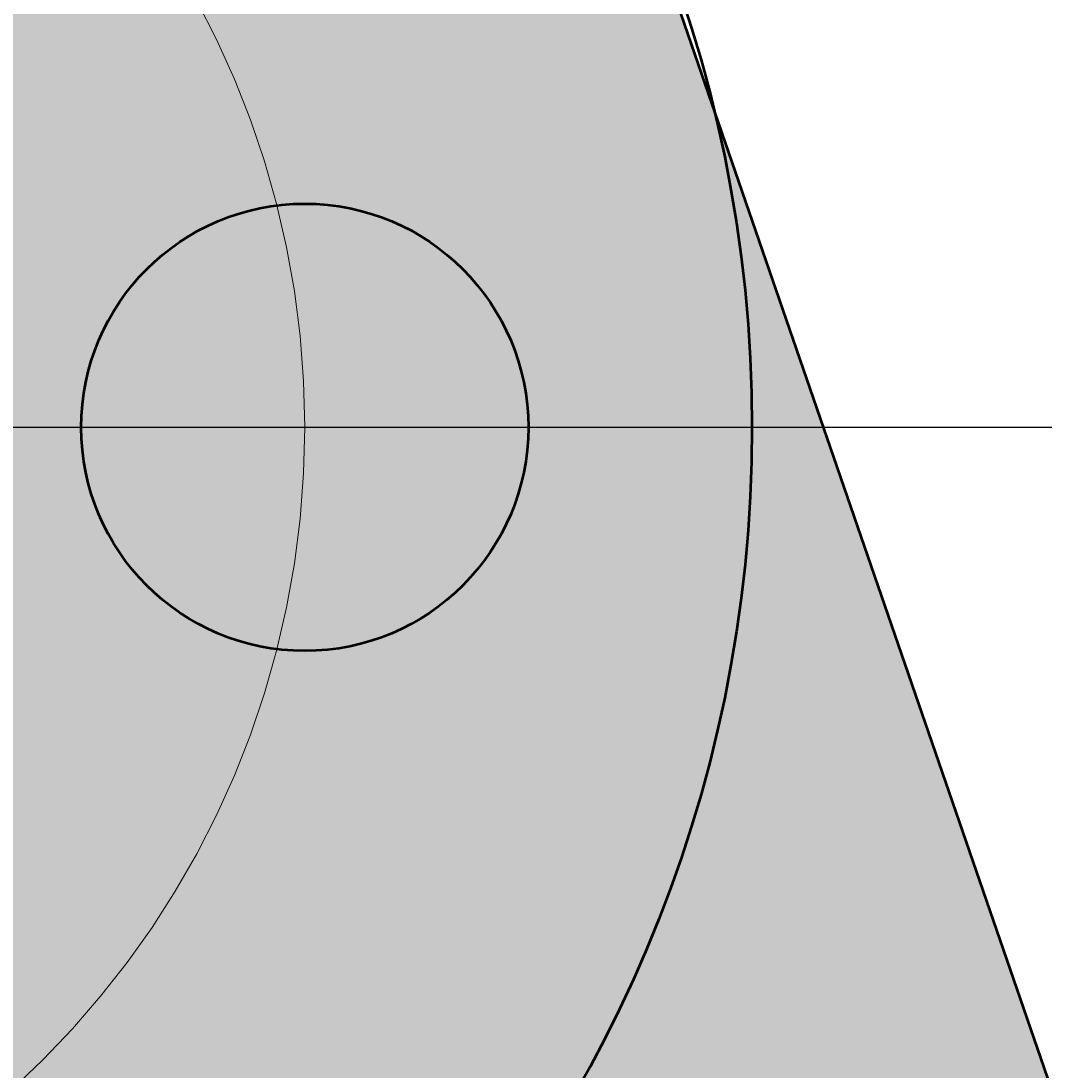
# Model space of a CAD drawing. Units: inches. Extents: x 114 to 236, y -51 to 115.
# Tile 12 of 14: x 189 to 212, y 65 to 88. Entities that reach past the tile are written whole.
import ezdxf

# ---------------------------------------------------------------- set-up
doc = ezdxf.new("R2010")
doc.units = ezdxf.units.IN
doc.header["$MEASUREMENT"] = 0
doc.linetypes.add('CENTER', pattern=[50.8, 31.75, -6.35, 6.35, -6.35])
for name, color, linetype, lineweight in [('M-CNTR', 7, 'CENTER', 18), ('M-DIMS', 2, 'Continuous', 18), ('M-OUTL', 7, 'Continuous', 50)]:
    doc.layers.add(name, color=color, linetype=linetype, lineweight=lineweight)
doc.layers.add('M-HATC', color=7, linetype='Continuous', lineweight=18, true_color=0xffffff)
doc.styles.get("Standard").update_dxf_attribs({"font": 'arial.ttf'})
doc.dimstyles.get("Standard").update_dxf_attribs({"dimtxt": 0.18, "dimasz": 0.18, "dimexe": 0.18, "dimexo": 0.0625, "dimgap": 0.09, "dimtad": 0, "dimtih": 1, "dimtoh": 1, "dimdec": 4, "dimzin": 0, "dimdsep": 46, "dimtxsty": 'Standard', "dimcen": 0.09, "dimadec": 0, "dimazin": 0, "dimtfac": 1, "dimtdec": 4, "dimtofl": 0, "dimtmove": 0, "dimatfit": 3, "dimfxl": 1, "dimtolj": 1, "dimtzin": 0, "dimarcsym": 0})

# ---------------------------------------------------------------- blocks, each defined once
blk = doc.blocks.new('BOLT-HOLE-D10')
blk.add_circle((0, 0), 5)
blk = doc.blocks.new('*D3')
at = {"layer": 'Defpoints', "color": 0, "transparency": 16777216}
for p in [(230.229, 115.287), (120.229, 9.307), (230.229, 9.307)]:
    blk.add_point(p, dxfattribs=at)
at = {"layer": 'M-DIMS', "color": 0, "lineweight": -2, "transparency": 16777216}
for p, q in [((120.229, 9.37), (120.229, 115.467)), ((120.409, 115.287), (174.949, 115.287)), ((230.049, 115.287), (175.509, 115.287)), ((230.229, 9.37), (230.229, 115.467))]:
    blk.add_line(p, q, dxfattribs=at)
at = {"layer": 'M-DIMS', "color": 0, "transparency": 16777216}
for points in [[(120.409, 115.317), (120.409, 115.257), (120.229, 115.287)], [(230.049, 115.317), (230.049, 115.257), (230.229, 115.287)]]:
    blk.add_solid(points, dxfattribs=at)
at = {"layer": 'M-DIMS', "color": 0, "transparency": 16777216, "insert": (175.229, 115.287), "char_height": 0.18, "attachment_point": 5}
blk.add_mtext('\\A1;110', dxfattribs=at)
blk = doc.blocks.new('*D6')
at = {"layer": 'Defpoints', "color": 0, "transparency": 16777216}
for p in [(175.229, 79.307), (215.229, 9.307), (215.229, -11.673)]:
    blk.add_point(p, dxfattribs=at)
at = {"layer": 'M-DIMS', "color": 0, "lineweight": -2, "transparency": 16777216}
for p, q in [((175.229, 79.245), (175.229, -11.853)), ((215.229, 9.245), (215.229, -11.853)), ((175.409, -11.673), (195.006, -11.673)), ((215.049, -11.673), (195.451, -11.673))]:
    blk.add_line(p, q, dxfattribs=at)
at = {"layer": 'M-DIMS', "color": 0, "transparency": 16777216}
for points in [[(175.409, -11.643), (175.409, -11.703), (175.229, -11.673)], [(215.049, -11.643), (215.049, -11.703), (215.229, -11.673)]]:
    blk.add_solid(points, dxfattribs=at)
at = {"layer": 'M-DIMS', "color": 0, "transparency": 16777216, "insert": (195.229, -11.673), "char_height": 0.18, "attachment_point": 5}
blk.add_mtext('\\A1;40', dxfattribs=at)
blk = doc.blocks.new('*D7')
at = {"layer": 'Defpoints', "color": 0, "transparency": 16777216}
for p in [(175.229, 79.307), (236.209, 79.307), (215.229, 9.307)]:
    blk.add_point(p, dxfattribs=at)
at = {"layer": 'M-DIMS', "color": 0, "lineweight": -2, "transparency": 16777216}
for p, q in [((175.291, 79.307), (236.389, 79.307)), ((236.209, 79.127), (236.209, 44.489)), ((236.209, 9.487), (236.209, 44.125)), ((215.291, 9.307), (236.389, 9.307))]:
    blk.add_line(p, q, dxfattribs=at)
at = {"layer": 'M-DIMS', "color": 0, "transparency": 16777216}
for points in [[(236.179, 79.127), (236.239, 79.127), (236.209, 79.307)], [(236.179, 9.487), (236.239, 9.487), (236.209, 9.307)]]:
    blk.add_solid(points, dxfattribs=at)
at = {"layer": 'M-DIMS', "color": 0, "transparency": 16777216, "insert": (236.209, 44.307), "char_height": 0.18, "attachment_point": 5}
blk.add_mtext('\\A1;70', dxfattribs=at)
blk = doc.blocks.new('*D8')
at = {"layer": 'Defpoints', "color": 0, "transparency": 16777216}
for p in [(197.149, 99.789), (153.308, 58.825)]:
    blk.add_point(p, dxfattribs=at)
at = {"layer": 'M-DIMS', "color": 0, "lineweight": -2, "transparency": 16777216}
for p, q in [((210.301, 112.078), (197.28, 99.912)), ((210.481, 112.078), (210.301, 112.078)), ((175.229, 79.217), (175.229, 79.397)), ((175.139, 79.307), (175.319, 79.307))]:
    blk.add_line(p, q, dxfattribs=at)
at = {"layer": 'M-DIMS', "color": 0, "transparency": 16777216}
blk.add_solid([(197.26, 99.934), (197.301, 99.89), (197.149, 99.789)], dxfattribs=at)
at = {"layer": 'M-DIMS', "color": 0, "transparency": 16777216, "insert": (210.797, 112.078), "char_height": 0.18, "attachment_point": 5}
blk.add_mtext('\\A1;∅60', dxfattribs=at)
blk = doc.blocks.new('*D9')
at = {"layer": 'Defpoints', "color": 0, "transparency": 16777216}
for p in [(157.908, 89.307), (192.549, 69.307)]:
    blk.add_point(p, dxfattribs=at)
at = {"layer": 'M-DIMS', "color": 0, "lineweight": -2, "transparency": 16777216}
for p, q in [((147.336, 95.307), (147.516, 95.307)), ((147.516, 95.307), (157.752, 89.397)), ((175.229, 79.217), (175.229, 79.397)), ((175.139, 79.307), (175.319, 79.307))]:
    blk.add_line(p, q, dxfattribs=at)
at = {"layer": 'M-DIMS', "color": 0, "transparency": 16777216}
blk.add_solid([(157.767, 89.423), (157.737, 89.371), (157.908, 89.307)], dxfattribs=at)
at = {"layer": 'M-DIMS', "color": 0, "transparency": 16777216, "insert": (147.019, 95.307), "char_height": 0.18, "attachment_point": 5}
blk.add_mtext('\\A1;∅40', dxfattribs=at)

msp = doc.modelspace()

# ---------------------------------------------------------------- hatches: boundary and pattern name
at = {"layer": 'M-HATC'}
h = msp.add_hatch(color=256, dxfattribs=at)
h.set_gradient(color1=(19, 155, 72), color2=(255, 255, 0), tint=1, name='HEMISPHERICAL')
h.paths.add_polyline_path([(147.853, 91.577), (146.105, 86.505, 0.060651), (145.229, 79.307, 1), (205.229, 79.307, 0.060651), (204.352, 86.505), (202.605, 91.577, 0.647643)])
h.paths.add_polyline_path([(180.229, 99.307, -0.031342), (180.189, 98.682, -0.27393), (194.604, 84.268, -0.451416), (200.229, 79.307, -0.451416), (194.604, 74.346, -0.27393), (180.189, 59.932, -0.031342), (180.229, 59.307, -1), (170.229, 59.307, -0.031342), (170.268, 59.932, -0.27393), (155.854, 74.346, -0.451416), (150.229, 79.307, -0.451416), (155.854, 84.268, -0.27393), (170.268, 98.682, -0.031342), (170.229, 99.307, -1)], flags=16)
h.paths.add_polyline_path([(183.229, 79.307, -1), (167.229, 79.307, -1)], flags=0)
h.paths.add_polyline_path([(155.854, 84.268, -0.377964), (160.229, 79.307, -0.377964), (155.854, 74.346, 0.27393), (170.268, 59.932, -0.881917), (180.189, 59.932, 0.27393), (194.604, 74.346, -0.377964), (190.229, 79.307, -0.377964), (194.604, 84.268, 0.27393), (180.189, 98.682, -0.881917), (170.268, 98.682, 0.27393)], flags=0)
h = msp.add_hatch(color=256, dxfattribs=at)
h.set_gradient(color1=(242, 103, 34), color2=(255, 255, 0), tint=1, name='INVSPHERICAL')
h.paths.add_polyline_path([(145.229, 79.307, -0.060651), (146.105, 86.505), (121.823, 16.038, -0.790743), (150.229, 9.307, -0.236068), (144.229, -2.693, -0.14094), (175.229, 9.098, -0.14094), (206.229, -2.693, -0.236068), (200.229, 9.307, -0.790743), (228.634, 16.038), (204.352, 86.505, -0.060651), (205.229, 79.307, -1)])
h = msp.add_hatch(color=256, dxfattribs=at)
h.paths.add_polyline_path([(195.229, 79.307, 0.062746), (194.604, 84.268, 0.377964), (190.229, 79.307, 0.377964), (194.604, 74.346, 0.062746)])
h.paths.add_polyline_path([(200.229, 79.307, 0.451416), (194.604, 84.268, -0.062746), (195.229, 79.307, -0.062746), (194.604, 74.346, 0.451416)])

# ---------------------------------------------------------------- linework, layer by layer
at = {"layer": 'M-CNTR'}
msp.add_circle((175.229, 79.307), 20, dxfattribs=at)
at = {"layer": 'M-OUTL'}
msp.add_line((229.935, 12.263), (202.605, 91.577), dxfattribs=at)
msp.add_circle((175.229, 79.307), 30, dxfattribs=at)

# ---------------------------------------------------------------- block references
msp.add_blockref('BOLT-HOLE-D10', (195.229, 79.307), dxfattribs=at)

# ---------------------------------------------------------------- dimensions: what is measured, and where the dimension line sits
at = {"layer": 'M-DIMS'}
for base, p1, p2, picture, middle in [((230.229, 115.287), (120.229, 9.307), (230.229, 9.307), '*D3', (175.229, 115.287)), ((215.229, -11.673), (175.229, 79.307), (215.229, 9.307), '*D6', (195.229, -11.673))]:
    dim = msp.add_linear_dim(base=base, p1=p1, p2=p2, dimstyle='Standard', override={"dimdec": 0, "dimlfac": 1, "dimrnd": 0, "dimzin": 0, "dimdsep": 46, "dimlunit": 2}, dxfattribs=at)
    dim.commit()
    dim.dimension.update_dxf_attribs({"geometry": picture, "text_midpoint": middle})
for p1, p2, picture, middle in [((153.308, 58.825), (197.149, 99.789), '*D8', (210.797, 112.078)), ((192.549, 69.307), (157.908, 89.307), '*D9', (147.019, 95.307))]:
    dim = msp.add_diameter_dim_2p(p1=p1, p2=p2, dimstyle='Standard', override={"dimdec": 0, "dimlfac": 1, "dimrnd": 0, "dimzin": 0, "dimdsep": 46, "dimlunit": 2}, dxfattribs=at)
    dim.commit()
    dim.dimension.update_dxf_attribs({"geometry": picture, "text_midpoint": middle, "dimtype": 163})
dim = msp.add_linear_dim(base=(236.209, 79.307), p1=(215.229, 9.307), p2=(175.229, 79.307), angle=90, dimstyle='Standard', override={"dimdec": 0, "dimlfac": 1, "dimrnd": 0, "dimzin": 0, "dimdsep": 46, "dimlunit": 2}, dxfattribs=at)
dim.commit()
dim.dimension.update_dxf_attribs({"geometry": '*D7', "text_midpoint": (236.209, 44.307)})

doc.saveas('drawing.dxf')
